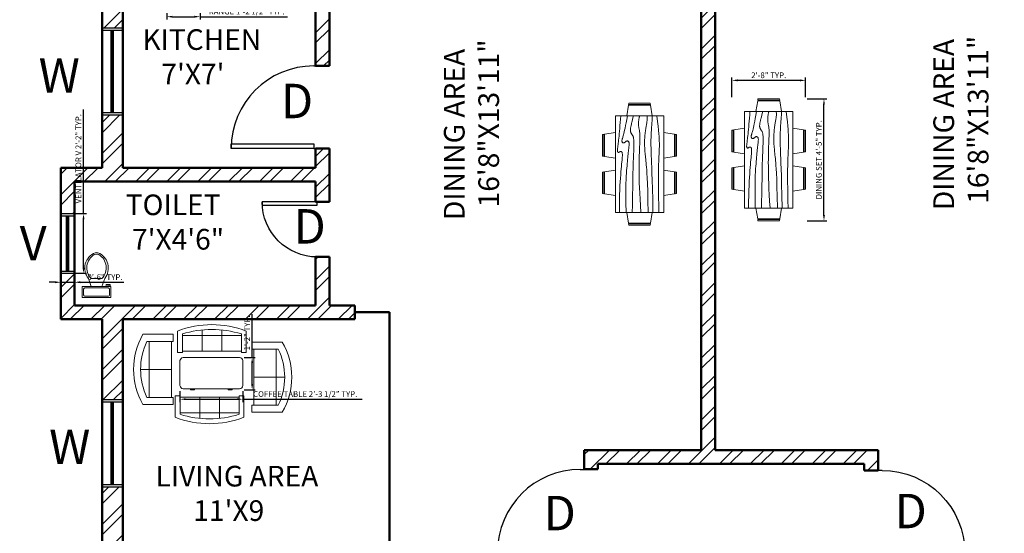
# Model space of a CAD drawing. Units: inches. Extents: x -31485 to -28799, y 18003 to 19130.
# Tile 12 of 15: x -29700 to -29271, y 18380 to 18604. Entities that reach past the tile are written whole.
import ezdxf

# ---------------------------------------------------------------- set-up
doc = ezdxf.new("R2010")
doc.units = ezdxf.units.IN
for name, color, linetype, lineweight in [('A-ANNO-DIMS', 2, 'Continuous', 18), ('A-ANNO-TEXT', 7, 'Continuous', 18), ('A-AREA-IDEN', 7, 'Continuous', 18), ('A-DOOR', 3, 'Continuous', 25), ('A-FLOR-FIXT', 9, 'Continuous', 18), ('A-FURN', 8, 'Continuous', 18), ('A-GLAZ', 4, 'Continuous', 25), ('A-WALL', 7, 'Continuous', 50), ('A-WALL-PATT', 8, 'Continuous', 13)]:
    doc.layers.add(name, color=color, linetype=linetype, lineweight=lineweight)
doc.styles.get("Standard").update_dxf_attribs({"font": 'arial.ttf'})
doc.dimstyles.new('ISO-25', dxfattribs={"dimtxt": 2.5, "dimasz": 2.5, "dimexe": 1.25, "dimexo": 0.625, "dimtad": 1, "dimdec": 0, "dimlunit": 3, "dimtxsty": 'Standard', "dimcen": 2.5, "dimadec": 0, "dimazin": 0, "dimtfac": 1, "dimtdec": 0, "dimtmove": 0, "dimatfit": 3, "dimfxl": 1, "dimarcsym": 0})

# ---------------------------------------------------------------- blocks, each defined once
blk = doc.blocks.new('*U8')
for p, q in [((0, 0), (0, -100)), ((750, 0), (750, -100))]:
    blk.add_line(p, q)
blk.add_lwpolyline([(0, 0), (0, 750), (43.75, 750), (43.75, 0)], close=True)
blk.add_arc((0, 0), 750, 0, 90)
blk = doc.blocks.new('Toilet - top')
for p, q in [((9.5, -6), (9.5, -2)), ((-10, -8.5), (-8, -8.5)), ((-10, -9.5), (-10, -8.5)), ((-7, -9.5), (-10, -9.5)), ((-8, -8.5), (-8, -8)), ((-7, -8), (-7, -9.5)), ((-4, -8), (-6, -14)), ((4, -14), (-4, -14)), ((4, -8), (6, -14))]:
    blk.add_line(p, q)
blk.add_lwpolyline([(10.5, -8), (10.5, 0), (-10.5, 0), (-10.5, -8)], close=True)
for points in [[(-9.5, -2), (-9.5, -6)], [(8.5, -1), (-8.5, -1)], [(-8.5, -7), (8.5, -7)]]:
    blk.add_lwpolyline(points)
for centre, radius, start, end in [((-8.62, -1.88), 0.884, 81.8699, 188.1301), ((-8.62, -6.12), 0.884, 171.8699, 278.1301), ((8.62, -1.88), 0.884, 351.8699, 98.1301), ((8.62, -6.12), 0.884, 261.8699, 8.1301), ((3.52, -21.58), 12.17, 141.46911, 247.97143), ((4.2, -21.82), 11.33, 136.36773, 238.94682), ((-3.52, -21.58), 12.17, 292.02843, 38.53071), ((-4.2, -21.82), 11.33, 301.05301, 43.63209), ((0, -27.88), 4, 245.73182, 294.26817), ((0, -29), 4, 254.86053, 285.13947)]:
    blk.add_arc(centre, radius, start, end)
blk = doc.blocks.new('Dining Set - 36 x 72 in.')
for p, q in [((-22.2343, 26.00059), (-23.4847, 17.99762)), ((-22.2304, 26), (-5.7608, 26)), ((-22, 27.5), (-22.1562, 26.50042)), ((-5.8416, 26.5), (-22.1534, 26.5)), ((-22, 27.5), (-6, 27.5)), ((-5.8437, 26.49966), (-6, 27.5)), ((-4.5152, 17.99762), (-5.7655, 25.99926)), ((5.7657, 26.00059), (4.5153, 17.99762)), ((5.7696, 26), (22.2392, 26)), ((6, 27.5), (5.8438, 26.50042)), ((22.1584, 26.5), (5.8466, 26.5)), ((6, 27.5), (22, 27.5)), ((22.1563, 26.49966), (22, 27.5)), ((23.4848, 17.99762), (22.2345, 25.99926)), ((36, 18), (-36, 18)), ((-36, 18), (-36, -18)), ((36, -18), (36, 18)), ((-45.5, 8), (-44.5004, 8.15617)), ((-45.5, 8), (-45.5, -8)), ((-44.5, -8.15843), (-44.5, 8.15338)), ((-44.0006, 8.23428), (-35.9976, 9.48474)), ((-44, 8.23041), (-44, -8.23915)), ((44.0006, 8.23428), (35.9976, 9.48474)), ((44, 8.23041), (44, -8.23915)), ((44.5, -8.15843), (44.5, 8.15338)), ((45.5, 8), (44.5005, 8.15617)), ((45.5, 8), (45.5, -8)), ((-44.4997, -8.15631), (-45.5, -8)), ((-35.9976, -9.48476), (-43.9993, -8.2345)), ((35.9976, -9.48476), (43.9993, -8.2345)), ((44.4997, -8.15631), (45.5, -8)), ((-36, -18), (36, -18)), ((-22.2343, -26.0006), (-23.4847, -17.99762)), ((-4.5152, -17.99762), (-5.7655, -25.99928)), ((5.7657, -26.0006), (4.5153, -17.99762)), ((23.4848, -17.99762), (22.2345, -25.99928)), ((-22.2304, -26), (-5.7608, -26)), ((-22, -27.5), (-22.1562, -26.50044)), ((-5.8416, -26.5), (-22.1534, -26.5)), ((-22, -27.5), (-6, -27.5)), ((-5.8437, -26.49967), (-6, -27.5)), ((5.7696, -26), (22.2392, -26)), ((6, -27.5), (5.8438, -26.50044)), ((22.1584, -26.5), (5.8466, -26.5)), ((6, -27.5), (22, -27.5)), ((22.1563, -26.49967), (22, -27.5))]:
    blk.add_line(p, q)
for points in [[(-36, 15), (-31.1772, 14.97754), (-26.8079, 14.91406), (-22.8538, 14.81543), (-19.276, 14.6875), (-16.0362, 14.53613), (-13.0957, 14.36718), (-10.4159, 14.18652), (-7.9583, 14), (-5.6904, 13.81315), (-3.6035, 13.63021), (-1.6954, 13.45508), (0.0365, 13.29166), (1.5945, 13.14388), (2.9811, 13.01562), (4.1988, 12.9108), (5.25, 12.83333), (6.1393, 12.78613), (6.8802, 12.76823), (7.4883, 12.77767), (7.9792, 12.8125), (8.3685, 12.87077), (8.6719, 12.95052), (8.9049, 13.0498), (9.0833, 13.16666), (9.2205, 13.29899), (9.3216, 13.44401), (9.3895, 13.59879), (9.4271, 13.76041), (9.4373, 13.92594), (9.4232, 14.09245), (9.3875, 14.257), (9.3333, 14.41666), (9.2638, 14.56917), (9.1836, 14.71484), (9.0975, 14.85465), (9.0104, 14.98958), (8.9272, 15.1206), (8.8529, 15.2487), (8.7922, 15.37483), (8.75, 15.5), (8.7305, 15.62467), (8.7344, 15.74739), (8.7617, 15.86621), (8.8125, 15.97916), (8.8867, 16.08431), (8.9844, 16.17968), (9.1055, 16.26334), (9.25, 16.33333), (9.4189, 16.38802), (9.6172, 16.42708), (9.8506, 16.45052), (10.125, 16.45833), (10.4463, 16.45052), (10.8203, 16.42708), (11.2529, 16.38802), (11.75, 16.33333), (12.3184, 16.26318), (12.9694, 16.17838), (13.7151, 16.07991), (14.5677, 15.96875), (15.5395, 15.84586), (16.6426, 15.71224), (17.8893, 15.56884), (19.2917, 15.41666), (20.859, 15.25667), (22.5879, 15.08984), (24.4721, 14.91715), (26.5052, 14.73958), (28.6809, 14.5581), (30.9929, 14.3737), (33.4347, 14.18733), (36, 14)], [(-36, 10), (-28.9766, 10.14274), (-23.1725, 10.20442), (-18.4241, 10.19775), (-14.5677, 10.13541), (-11.4399, 10.03011), (-8.877, 9.89453), (-6.7154, 9.74137), (-4.7917, 9.58333), (-2.9698, 9.43082), (-1.2246, 9.28515), (0.4415, 9.14534), (2.026, 9.01041), (3.5266, 8.87939), (4.9408, 8.7513), (6.266, 8.62516), (7.5, 8.5), (8.6411, 8.37549), (9.6914, 8.2539), (10.6538, 8.13818), (11.5312, 8.03125), (12.3267, 7.93603), (13.043, 7.85547), (13.6831, 7.79248), (14.25, 7.75), (14.7471, 7.7303), (15.1797, 7.73307), (15.5537, 7.75732), (15.875, 7.80208), (16.1494, 7.86637), (16.3828, 7.94922), (16.5811, 8.04964), (16.75, 8.16666), (16.8944, 8.29915), (17.0143, 8.44531), (17.1089, 8.60319), (17.1771, 8.77083), (17.218, 8.94629), (17.2305, 9.1276), (17.2137, 9.31282), (17.1667, 9.5), (17.0895, 9.6875), (16.987, 9.875), (16.8649, 10.0625), (16.7292, 10.25), (16.5856, 10.4375), (16.4401, 10.625), (16.2985, 10.8125), (16.1667, 11), (16.05, 11.18733), (15.9518, 11.3737), (15.8752, 11.5581), (15.8229, 11.73958), (15.798, 11.91715), (15.8034, 12.08984), (15.842, 12.25667), (15.9167, 12.41666), (16.0295, 12.56836), (16.1784, 12.70833), (16.3605, 12.83268), (16.5729, 12.9375), (16.8127, 13.01888), (17.0768, 13.07291), (17.3625, 13.0957), (17.6667, 13.08333), (17.9894, 13.03312), (18.3418, 12.94726), (18.7382, 12.82918), (19.1927, 12.68229), (19.7195, 12.51001), (20.3327, 12.31575), (21.0465, 12.10294), (21.875, 11.875), (22.8357, 11.63354), (23.959, 11.37304), (25.2786, 11.08618), (26.8282, 10.76562), (28.6414, 10.40405), (30.752, 9.99414), (33.1936, 9.52856), (36, 9)], [(-36, 5.5), (-30.7157, 5.3348), (-26.069, 5.20963), (-21.9946, 5.11767), (-18.4271, 5.05208), (-15.3009, 5.00602), (-12.5508, 4.97265), (-10.1112, 4.94515), (-7.9167, 4.91666), (-5.909, 4.88167), (-4.0586, 4.83984), (-2.3429, 4.79215), (-0.7396, 4.73958), (0.7739, 4.6831), (2.22, 4.6237), (3.6213, 4.56233), (5, 4.5), (6.373, 4.43782), (7.7344, 4.3776), (9.0723, 4.32129), (10.375, 4.27083), (11.6309, 4.22819), (12.8281, 4.19531), (13.9551, 4.17415), (15, 4.16666), (15.954, 4.17448), (16.819, 4.19791), (17.6001, 4.23698), (18.3021, 4.29166), (18.9299, 4.36198), (19.4883, 4.44791), (19.9823, 4.54948), (20.4167, 4.66666), (20.7969, 4.79899), (21.1302, 4.94401), (21.4245, 5.09879), (21.6875, 5.26041), (21.9271, 5.42594), (22.1511, 5.59245), (22.3672, 5.757), (22.5834, 5.91666), (22.8065, 6.06868), (23.0404, 6.21093), (23.2879, 6.34147), (23.5521, 6.45833), (23.8358, 6.55957), (24.142, 6.64323), (24.4735, 6.70735), (24.8334, 6.75), (25.2235, 6.76969), (25.642, 6.76692), (26.0858, 6.74267), (26.5521, 6.69791), (27.0379, 6.63362), (27.5404, 6.55078), (28.0565, 6.45036), (28.5834, 6.33333), (29.1242, 6.19987), (29.7071, 6.04687), (30.3661, 5.87044), (31.1354, 5.66666), (32.0493, 5.43164), (33.142, 5.16146), (34.4475, 4.85221), (36, 4.5)], [(-36, -1), (-30.7915, -0.6591), (-26.0195, -0.38216), (-21.6519, -0.16284), (-17.6563, 0.00521), (-14.0005, 0.12833), (-10.6523, 0.21289), (-7.5796, 0.26522), (-4.75, 0.29166), (-2.134, 0.29793), (0.2878, 0.28711), (2.5317, 0.26163), (4.6146, 0.22396), (6.5529, 0.17651), (8.3633, 0.12174), (10.0623, 0.06209), (11.6667, 0), (13.1899, -0.06201), (14.6341, -0.1211), (15.9982, -0.17432), (17.2813, -0.21875), (18.4823, -0.25147), (19.6003, -0.26953), (20.6343, -0.27002), (21.5834, -0.25), (22.4481, -0.20768), (23.2357, -0.14584), (23.9549, -0.06836), (24.6146, 0.02083), (25.2235, 0.11784), (25.7904, 0.21875), (26.3241, 0.31966), (26.8334, 0.41666), (27.3265, 0.50618), (27.8099, 0.58593), (28.2894, 0.65397), (28.7709, 0.70833), (29.2601, 0.74707), (29.763, 0.76823), (30.2855, 0.76985), (30.8334, 0.75), (31.4088, 0.70784), (31.9994, 0.64713), (32.589, 0.57275), (33.1615, 0.48958), (33.7008, 0.4025), (34.1908, 0.3164), (34.6153, 0.23616), (34.9584, 0.16666), (35.2099, 0.11165), (35.3848, 0.07031), (35.504, 0.04069), (35.5886, 0.02083), (35.6594, 0.00879), (35.7377, 0.0026), (35.8442, 0.00032), (36, 0)], [(-36, -6.5), (-27.1843, -6.31267), (-20.084, -6.1263), (-14.469, -5.9419), (-10.1094, -5.76042), (-6.7752, -5.58285), (-4.2363, -5.41016), (-2.2629, -5.24333), (-0.625, -5.08334), (0.8708, -4.93099), (2.2715, -4.78646), (3.5872, -4.64974), (4.8281, -4.52084), (6.0046, -4.39974), (7.127, -4.28646), (8.2053, -4.18099), (9.25, -4.08334), (10.2705, -3.99382), (11.2734, -3.91407), (12.2647, -3.84603), (13.25, -3.79167), (14.2354, -3.75293), (15.2266, -3.73177), (16.2295, -3.73015), (17.25, -3.75), (18.2912, -3.79248), (19.3451, -3.85547), (20.4009, -3.93604), (21.4479, -4.03125), (22.4754, -4.13819), (23.4727, -4.25391), (24.4289, -4.37549), (25.3334, -4.5), (26.1785, -4.62492), (26.9694, -4.74935), (27.7145, -4.87281), (28.4219, -4.99479), (29.1, -5.11483), (29.7572, -5.23242), (30.4016, -5.34709), (31.0417, -5.45834), (31.6837, -5.56437), (32.3262, -5.65821), (32.9658, -5.73153), (33.599, -5.77604), (34.2224, -5.78345), (34.8327, -5.74545), (35.4264, -5.65373), (36, -5.5)], [(-36, -10), (-26.4022, -9.81299), (-18.4675, -9.62891), (-11.9839, -9.45069), (-6.7396, -9.28125), (-2.5226, -9.12354), (0.8789, -8.98047), (3.6769, -8.85498), (6.0833, -8.75), (8.2767, -8.66765), (10.3021, -8.60677), (12.1712, -8.56543), (13.8958, -8.54167), (15.4876, -8.53353), (16.9583, -8.53907), (18.3197, -8.55632), (19.5834, -8.58334), (20.7616, -8.61841), (21.8685, -8.66081), (22.9188, -8.71004), (23.9271, -8.76563), (24.9081, -8.82707), (25.8763, -8.89388), (26.8465, -8.96558), (27.8334, -9.04167), (28.8474, -9.12118), (29.8828, -9.20117), (30.93, -9.27824), (31.9792, -9.34896), (33.0205, -9.40991), (34.0443, -9.45768), (35.0407, -9.48885), (36, -9.5)], [(-36, -14.5), (-30.0881, -14.33513), (-25.0332, -14.21224), (-20.7312, -14.12647), (-17.0781, -14.07292), (-13.97, -14.04671), (-11.3027, -14.04297), (-8.9724, -14.05681), (-6.875, -14.08334), (-4.9224, -14.11833), (-3.0905, -14.16016), (-1.3709, -14.20785), (0.2448, -14.26042), (1.7647, -14.3169), (3.1973, -14.3763), (4.5507, -14.43767), (5.8333, -14.5), (7.0554, -14.5621), (8.235, -14.62175), (9.3922, -14.67652), (10.5469, -14.72396), (11.7192, -14.76164), (12.929, -14.78711), (14.1965, -14.79794), (15.5417, -14.79167), (16.9933, -14.76424), (18.6152, -14.70508), (20.4804, -14.60197), (22.6615, -14.44271), (25.2312, -14.21509), (28.2624, -13.9069), (31.8277, -13.50594), (36, -13)]]:
    blk.add_lwpolyline(points)
blk = doc.blocks.new('Desk - 30 x 60 in.')
for p, q in [((-26.999995, 0), (26.999995, 0)), ((-29.999995, -27), (-29.999995, -3)), ((29.999995, -3), (29.999995, -27)), ((26.999995, -30), (-26.999995, -30)), ((-20.000005, -30), (-20.000005, -31)), ((-20.000005, -31), (-16.000005, -31)), ((-16.000005, -31), (-16.000005, -30)), ((15.999995, -31), (15.999995, -30)), ((19.999995, -31), (15.999995, -31)), ((19.999995, -30), (19.999995, -31))]:
    blk.add_line(p, q)
for centre, start, end in [((-26.499995, -3.5), 98.1301, 171.8699), ((26.499995, -3.5), 8.130102, 81.8699), ((-26.499995, -26.5), 188.1301, 261.8699), ((26.499995, -26.5), 278.1301, 351.8699)]:
    blk.add_arc(centre, 3.535534, start, end)
blk = doc.blocks.new('Sofa - Roundback 7 ft.')
for p, q in [((-36.000027, -34), (-36.000027, -11.4696)), ((-12.00002, -32.4421), (-12.00003, -6.5971)), ((11.99997, -32.4421), (11.99998, -6.5971)), ((35.99998, -34), (35.99998, -11.4696)), ((-35.999844, -13.3819), (35.9998, -13.3819)), ((-36.000027, -32.4421), (35.99998, -32.4421))]:
    blk.add_line(p, q)
for points in [[(-36.000027, -34), (-42.000027, -34), (-42.000027, -8)], [(41.99998, -8), (41.99998, -34), (35.99998, -34)]]:
    blk.add_lwpolyline(points)
for centre, radius, start, end in [((0, -114.25), 114.25, 68.43141, 111.5686), ((-0.00001, -127.1968), 121.1968, 72.72033, 107.2797)]:
    blk.add_arc(centre, radius, start, end)
blk = doc.blocks.new('Sofa - Roundback Loveseat 5 ft.')
for p, q in [((0, -32.44198), (0, -5.99998)), ((-24, -33.99998), (-24, -11.46958)), ((-23.9998, -13.38178), (23.99986, -13.38178)), ((24.00004, -33.99998), (24.00004, -11.46958)), ((-24, -32.44198), (24.00004, -32.44198))]:
    blk.add_line(p, q)
for points in [[(-24, -33.99998), (-30, -33.99998), (-30, -7.99998)], [(30.00004, -7.99998), (30.00004, -33.99998), (24.00004, -33.99998)]]:
    blk.add_lwpolyline(points)
for centre, radius, start, end in [((0, -60.24998), 60.24998, 60.13715, 119.8628), ((0, -61.38438), 55.38444, 64.32083, 115.6792)]:
    blk.add_arc(centre, radius, start, end)
blk = doc.blocks.new('WIN-900-W9')
for p, q in [((-29982.21, 18824.12), (-29982.21, 18815.12)), ((-29981.21, 18824.12), (-29981.21, 18815.12)), ((-29945.21, 18824.12), (-29945.21, 18815.12)), ((-29944.21, 18824.12), (-29944.21, 18815.12)), ((-29981.21, 18820.12), (-29945.21, 18820.12)), ((-29981.21, 18819.62), (-29945.21, 18819.62)), ((-29981.21, 18819.12), (-29945.21, 18819.12))]:
    blk.add_line(p, q)
blk = doc.blocks.new('VENT-600-W6')
for p, q in [((-29884.21, 18519.12), (-29878.21, 18519.12)), ((-29884.21, 18518.12), (-29878.21, 18518.12)), ((-29881.71, 18494.12), (-29881.71, 18518.12)), ((-29881.21, 18494.12), (-29881.21, 18518.12)), ((-29880.71, 18494.12), (-29880.71, 18518.12)), ((-29884.21, 18494.12), (-29878.21, 18494.12)), ((-29884.21, 18493.12), (-29878.21, 18493.12))]:
    blk.add_line(p, q)
blk = doc.blocks.new('*D214')
at = {"layer": 'A-ANNO-DIMS', "color": 0, "lineweight": -2, "transparency": 16777216}
for p, q in [((-29671.92, 18519.12), (-29671.92, 18564.43)), ((-29675.2, 18519.12), (-29670.67, 18519.12)), ((-29671.92, 18495.62), (-29671.92, 18516.62)), ((-29675.2, 18493.12), (-29670.67, 18493.12))]:
    blk.add_line(p, q, dxfattribs=at)
at = {"layer": 'A-ANNO-DIMS', "color": 0, "transparency": 16777216}
for points in [[(-29672.34, 18516.62), (-29671.5, 18516.62), (-29671.92, 18519.12)], [(-29672.34, 18495.62), (-29671.5, 18495.62), (-29671.92, 18493.12)]]:
    blk.add_solid(points, dxfattribs=at)
at = {"layer": 'Defpoints', "color": 0, "transparency": 16777216}
for p in [(-29675.82, 18519.12), (-29671.92, 18519.12), (-29675.82, 18493.12)]:
    blk.add_point(p, dxfattribs=at)
at = {"layer": 'A-ANNO-DIMS', "color": 0, "transparency": 16777216, "insert": (-29673.84, 18543.02), "char_height": 2.5, "attachment_point": 5, "rotation": 90}
blk.add_mtext('VENTILATOR V 2\'-2" TYP.', dxfattribs=at)
blk = doc.blocks.new('*D215')
at = {"layer": 'A-ANNO-DIMS', "color": 0, "lineweight": -2, "transparency": 16777216}
for p, q in [((-29681.82, 18492.49), (-29681.82, 18487.97)), ((-29675.82, 18492.49), (-29675.82, 18487.97)), ((-29684.32, 18489.22), (-29686.82, 18489.22)), ((-29681.82, 18489.22), (-29675.82, 18489.22)), ((-29673.32, 18489.22), (-29654.33, 18489.22))]:
    blk.add_line(p, q, dxfattribs=at)
at = {"layer": 'A-ANNO-DIMS', "color": 0, "transparency": 16777216}
for points in [[(-29684.32, 18489.63), (-29684.32, 18488.8), (-29681.82, 18489.22)], [(-29673.32, 18489.63), (-29673.32, 18488.8), (-29675.82, 18489.22)]]:
    blk.add_solid(points, dxfattribs=at)
at = {"layer": 'Defpoints', "color": 0, "transparency": 16777216}
for p in [(-29681.82, 18493.12), (-29675.82, 18493.12), (-29675.82, 18489.22)]:
    blk.add_point(p, dxfattribs=at)
at = {"layer": 'A-ANNO-DIMS', "color": 0, "transparency": 16777216, "insert": (-29662.58, 18491.12), "char_height": 2.5, "attachment_point": 5}
blk.add_mtext('0\'-6" TYP.', dxfattribs=at)
blk = doc.blocks.new('*D244')
at = {"layer": 'A-ANNO-DIMS', "color": 0, "lineweight": -2, "transparency": 16777216}
for p, q in [((-29629.9, 18441.75), (-29629.9, 18437.02)), ((-29602.57, 18441.75), (-29602.57, 18437.02)), ((-29627.4, 18438.27), (-29605.07, 18438.27)), ((-29602.57, 18438.27), (-29550.61, 18438.27))]:
    blk.add_line(p, q, dxfattribs=at)
at = {"layer": 'A-ANNO-DIMS', "color": 0, "transparency": 16777216}
for points in [[(-29627.4, 18438.69), (-29627.4, 18437.86), (-29629.9, 18438.27)], [(-29605.07, 18438.69), (-29605.07, 18437.86), (-29602.57, 18438.27)]]:
    blk.add_solid(points, dxfattribs=at)
at = {"layer": 'Defpoints', "color": 0, "transparency": 16777216}
for p in [(-29629.9, 18442.37), (-29602.57, 18442.37), (-29602.57, 18438.27)]:
    blk.add_point(p, dxfattribs=at)
at = {"layer": 'A-ANNO-DIMS', "color": 0, "transparency": 16777216, "insert": (-29575.34, 18440.19), "char_height": 2.5, "attachment_point": 5}
blk.add_mtext('COFFEE TABLE 2\'-3 1/2" TYP.', dxfattribs=at)
blk = doc.blocks.new('*D245')
at = {"layer": 'A-ANNO-DIMS', "color": 0, "lineweight": -2, "transparency": 16777216}
for p, q in [((-29598.46, 18456.5), (-29598.46, 18475.25)), ((-29601.94, 18456.5), (-29597.21, 18456.5)), ((-29598.46, 18444.87), (-29598.46, 18454)), ((-29601.94, 18442.37), (-29597.21, 18442.37))]:
    blk.add_line(p, q, dxfattribs=at)
at = {"layer": 'A-ANNO-DIMS', "color": 0, "transparency": 16777216}
for points in [[(-29598.88, 18454), (-29598.05, 18454), (-29598.46, 18456.5)], [(-29598.88, 18444.87), (-29598.05, 18444.87), (-29598.46, 18442.37)]]:
    blk.add_solid(points, dxfattribs=at)
at = {"layer": 'Defpoints', "color": 0, "transparency": 16777216}
for p in [(-29602.57, 18456.5), (-29598.46, 18456.5), (-29602.57, 18442.37)]:
    blk.add_point(p, dxfattribs=at)
at = {"layer": 'A-ANNO-DIMS', "color": 0, "transparency": 16777216, "insert": (-29600.35, 18467.13), "char_height": 2.5, "attachment_point": 5, "rotation": 90}
blk.add_mtext('1\'-2" TYP.', dxfattribs=at)
blk = doc.blocks.new('*D250')
at = {"layer": 'A-ANNO-DIMS', "color": 0, "lineweight": -2, "transparency": 16777216}
for p, q in [((-29635.69, 18606.46), (-29635.69, 18603.66)), ((-29621.14, 18606.46), (-29621.14, 18603.66)), ((-29633.19, 18604.91), (-29623.64, 18604.91)), ((-29621.14, 18604.91), (-29583.06, 18604.91))]:
    blk.add_line(p, q, dxfattribs=at)
at = {"layer": 'A-ANNO-DIMS', "color": 0, "transparency": 16777216}
for points in [[(-29633.19, 18605.32), (-29633.19, 18604.49), (-29635.69, 18604.91)], [(-29623.64, 18605.32), (-29623.64, 18604.49), (-29621.14, 18604.91)]]:
    blk.add_solid(points, dxfattribs=at)
at = {"layer": 'Defpoints', "color": 0, "transparency": 16777216}
for p in [(-29635.69, 18607.09), (-29621.14, 18607.09), (-29621.14, 18604.91)]:
    blk.add_point(p, dxfattribs=at)
at = {"layer": 'A-ANNO-DIMS', "color": 0, "transparency": 16777216, "insert": (-29600.85, 18606.82), "char_height": 2.5, "attachment_point": 5}
blk.add_mtext('RANGE 1\'-2 1/2" TYP.', dxfattribs=at)
blk = doc.blocks.new('*D262')
at = {"layer": 'A-ANNO-DIMS', "color": 0, "lineweight": -2, "transparency": 16777216}
for p, q in [((-29356.73, 18569.18), (-29348.13, 18569.18)), ((-29349.38, 18518.47), (-29349.38, 18566.68)), ((-29356.73, 18515.97), (-29348.13, 18515.97))]:
    blk.add_line(p, q, dxfattribs=at)
at = {"layer": 'A-ANNO-DIMS', "color": 0, "transparency": 16777216}
for points in [[(-29349.79, 18566.68), (-29348.96, 18566.68), (-29349.38, 18569.18)], [(-29349.79, 18518.47), (-29348.96, 18518.47), (-29349.38, 18515.97)]]:
    blk.add_solid(points, dxfattribs=at)
at = {"layer": 'Defpoints', "color": 0, "transparency": 16777216}
for p in [(-29357.36, 18569.18), (-29349.38, 18569.18), (-29357.36, 18515.97)]:
    blk.add_point(p, dxfattribs=at)
at = {"layer": 'A-ANNO-DIMS', "color": 0, "transparency": 16777216, "insert": (-29351.3, 18542.58), "char_height": 2.5, "attachment_point": 5, "rotation": 90}
blk.add_mtext('DINING SET 4\'-5" TYP.', dxfattribs=at)
blk = doc.blocks.new('*D263')
at = {"layer": 'A-ANNO-DIMS', "color": 0, "lineweight": -2, "transparency": 16777216}
for p, q in [((-29389.52, 18569.81), (-29389.52, 18578.42)), ((-29359.86, 18577.17), (-29387.02, 18577.17)), ((-29357.36, 18569.81), (-29357.36, 18578.42))]:
    blk.add_line(p, q, dxfattribs=at)
at = {"layer": 'A-ANNO-DIMS', "color": 0, "transparency": 16777216}
for points in [[(-29387.02, 18577.58), (-29387.02, 18576.75), (-29389.52, 18577.17)], [(-29359.86, 18577.58), (-29359.86, 18576.75), (-29357.36, 18577.17)]]:
    blk.add_solid(points, dxfattribs=at)
at = {"layer": 'Defpoints', "color": 0, "transparency": 16777216}
for p in [(-29389.52, 18577.17), (-29389.52, 18569.18), (-29357.36, 18569.18)]:
    blk.add_point(p, dxfattribs=at)
at = {"layer": 'A-ANNO-DIMS', "color": 0, "transparency": 16777216, "insert": (-29373.44, 18579.07), "char_height": 2.5, "attachment_point": 5}
blk.add_mtext('2\'-8" TYP.', dxfattribs=at)

msp = doc.modelspace()

# ---------------------------------------------------------------- hatches: boundary and pattern name
at = {"layer": 'A-WALL-PATT'}
h = msp.add_hatch(dxfattribs=at)
h.set_pattern_fill('ANSI32', color=256)
h.set_pattern_definition([(45, (-227.67, 0), (-6.735192, 6.735192), []), (45, (-223.18, 0), (-6.735192, 6.735192), [])])
h.paths.add_polyline_path([(-29507.82, 18213.12), (-29493.82, 18213.12), (-29493.82, 18219.12), (-29507.82, 18219.12), (-29507.82, 18309.12), (-29504.3, 18309.12), (-29504.3, 18315.12), (-29513.82, 18315.12), (-29513.82, 18243.12), (-29654.82, 18243.12), (-29654.82, 18265.36), (-29663.82, 18265.36), (-29663.82, 18180.12), (-29603.32, 18180.12), (-29603.32, 18189.12), (-29654.82, 18189.12), (-29654.82, 18237.12), (-29513.82, 18237.12), (-29513.82, 18189.12), (-29565.32, 18189.12), (-29565.32, 18180.12), (-29507.82, 18180.12)])
h.paths.add_polyline_path([(-29408.82, 18189.12), (-29447.82, 18189.12), (-29447.82, 18371.74), (-29453.82, 18371.74), (-29453.82, 18365.12), (-29476.66, 18365.12), (-29476.66, 18359.12), (-29453.82, 18359.12), (-29453.82, 18315.12), (-29480.3, 18315.12), (-29480.3, 18309.12), (-29453.82, 18309.12), (-29453.82, 18219.12), (-29467.82, 18219.12), (-29467.82, 18213.12), (-29453.82, 18213.12), (-29453.82, 18180.12), (-29408.82, 18180.12)])
h.paths.add_polyline_path([(-29325.82, 18213.12), (-29311.82, 18213.12), (-29311.82, 18219.12), (-29325.82, 18219.12), (-29325.82, 18309.12), (-29298.35, 18309.12), (-29298.35, 18315.12), (-29325.82, 18315.12), (-29325.82, 18359.12), (-29304.41, 18359.12), (-29304.41, 18365.12), (-29325.82, 18365.12), (-29325.82, 18371.25), (-29331.82, 18371.25), (-29331.82, 18189.12), (-29370.82, 18189.12), (-29370.82, 18180.12), (-29325.82, 18180.12)])
h.paths.add_polyline_path([(-29265.82, 18237.12), (-29124.82, 18237.12), (-29124.82, 18189.12), (-29176.32, 18189.12), (-29176.32, 18180.12), (-29115.82, 18180.12), (-29115.82, 18268.84), (-29124.82, 18268.84), (-29124.82, 18243.12), (-29265.82, 18243.12), (-29265.82, 18315.12), (-29274.35, 18315.12), (-29274.35, 18309.12), (-29271.82, 18309.12), (-29271.82, 18219.12), (-29285.82, 18219.12), (-29285.82, 18213.12), (-29271.82, 18213.12), (-29271.82, 18180.12), (-29214.32, 18180.12), (-29214.32, 18189.12), (-29265.82, 18189.12)])
h.paths.add_polyline_path([(-29209.82, 18365.12), (-29262.82, 18365.12), (-29268.41, 18365.12), (-29268.41, 18359.12), (-29209.82, 18359.12)])
h.paths.add_polyline_path([(-29085.82, 18365.12), (-29115.82, 18365.12), (-29115.82, 18400.12), (-29124.82, 18400.12), (-29124.82, 18365.12), (-29171.82, 18365.12), (-29171.82, 18359.12), (-29124.82, 18359.12), (-29124.82, 18306.84), (-29115.82, 18306.84), (-29115.82, 18317.12), (-29085.82, 18317.12)])
h.paths.add_polyline_path([(-29115.82, 18359.12), (-29091.82, 18359.12), (-29091.82, 18323.12), (-29115.82, 18323.12)], flags=16)
h.paths.add_polyline_path([(-29607.82, 18365.12), (-29654.82, 18365.12), (-29654.82, 18400.12), (-29663.82, 18400.12), (-29663.82, 18365.12), (-29693.82, 18365.12), (-29693.82, 18317.12), (-29663.82, 18317.12), (-29663.82, 18303.36), (-29654.82, 18303.36), (-29654.82, 18359.12), (-29607.82, 18359.12)])
h.paths.add_polyline_path([(-29663.82, 18359.12), (-29663.82, 18323.12), (-29687.82, 18323.12), (-29687.82, 18359.12)], flags=16)
h.paths.add_polyline_path([(-29512.66, 18365.12), (-29516.82, 18365.12), (-29569.82, 18365.12), (-29569.82, 18359.12), (-29512.66, 18359.12)])
h.paths.add_polyline_path([(-29654.82, 18473.12), (-29553.73, 18473.12), (-29553.73, 18479.12), (-29564.82, 18479.12), (-29564.82, 18500.25), (-29569.57, 18500.25, -0.011537), (-29570.67, 18500.25), (-29570.82, 18500.25), (-29570.82, 18479.12), (-29675.82, 18479.12), (-29675.82, 18493.12), (-29681.82, 18493.12), (-29681.82, 18473.12), (-29663.82, 18473.12), (-29663.82, 18438.12), (-29654.82, 18438.12)])
h.paths.add_polyline_path([(-29564.82, 18547.44), (-29570.82, 18547.44), (-29570.82, 18539.12), (-29654.82, 18539.12), (-29654.82, 18562.12), (-29663.82, 18562.12), (-29663.82, 18539.12), (-29681.82, 18539.12), (-29681.82, 18519.12), (-29675.82, 18519.12), (-29675.82, 18533.12), (-29570.82, 18533.12), (-29570.82, 18524.25), (-29564.82, 18524.25)])
h.paths.add_polyline_path([(-29563.19, 18629.12), (-29654.82, 18629.12), (-29654.82, 18682.12), (-29663.82, 18682.12), (-29663.82, 18600.12), (-29654.82, 18600.12), (-29654.82, 18623.12), (-29570.82, 18623.12), (-29570.82, 18583.44), (-29566.85, 18583.44), (-29564.82, 18583.44), (-29564.82, 18623.12), (-29563.19, 18623.12)])
h.paths.add_polyline_path([(-29315.33, 18629.12), (-29396.82, 18629.12), (-29396.82, 18682.12), (-29402.82, 18682.12), (-29402.82, 18629.12), (-29482.28, 18629.12), (-29482.28, 18626.12), (-29482.28, 18623.12), (-29402.82, 18623.12), (-29402.82, 18416.12), (-29453.82, 18416.12), (-29453.82, 18407.74), (-29447.82, 18407.74), (-29447.82, 18410.12), (-29331.82, 18410.12), (-29331.82, 18407.25), (-29325.82, 18407.25), (-29325.82, 18416.12), (-29396.82, 18416.12), (-29396.82, 18623.12), (-29315.33, 18623.12)])
h.paths.add_polyline_path([(-29525.82, 18773.12), (-29492.32, 18773.12), (-29492.32, 18779.12), (-29498.82, 18779.12), (-29498.82, 18815.12), (-29469.82, 18815.12), (-29469.82, 18824.12), (-29504.82, 18824.12), (-29504.82, 18779.12), (-29552.82, 18779.12), (-29552.82, 18824.12), (-29587.82, 18824.12), (-29587.82, 18815.12), (-29558.82, 18815.12), (-29558.82, 18779.12), (-29563.08, 18779.12), (-29563.08, 18776.12), (-29563.08, 18773.12), (-29531.82, 18773.12), (-29531.82, 18629.12), (-29533.3, 18629.12), (-29533.3, 18626.12), (-29533.3, 18623.12), (-29518.28, 18623.12), (-29518.28, 18629.12), (-29525.82, 18629.12)])
h.paths.add_polyline_path([(-29654.82, 18779.12), (-29654.82, 18815.12), (-29625.82, 18815.12), (-29625.82, 18824.12), (-29663.82, 18824.12), (-29663.82, 18779.12), (-29693.82, 18779.12), (-29693.82, 18731.12), (-29663.82, 18731.12), (-29663.82, 18720.12), (-29654.82, 18720.12), (-29654.82, 18773.12), (-29587.08, 18773.12), (-29587.08, 18779.12)])
h.paths.add_polyline_path([(-29663.82, 18773.12), (-29663.82, 18737.12), (-29687.82, 18737.12), (-29687.82, 18773.12)], flags=16)
h.paths.add_polyline_path([(-29396.82, 18815.12), (-29367.82, 18815.12), (-29367.82, 18824.12), (-29431.82, 18824.12), (-29431.82, 18815.12), (-29402.82, 18815.12), (-29402.82, 18779.12), (-29468.32, 18779.12), (-29468.32, 18776.12), (-29468.32, 18773.12), (-29402.82, 18773.12), (-29402.82, 18720.12), (-29396.82, 18720.12), (-29396.82, 18773.12), (-29331.17, 18773.12), (-29331.17, 18779.12), (-29396.82, 18779.12)])
h.paths.add_polyline_path([(-29232.68, 18779.12), (-29240.82, 18779.12), (-29240.82, 18815.12), (-29201.82, 18815.12), (-29201.82, 18824.12), (-29246.82, 18824.12), (-29246.82, 18779.12), (-29294.82, 18779.12), (-29294.82, 18824.12), (-29329.82, 18824.12), (-29329.82, 18815.12), (-29300.82, 18815.12), (-29300.82, 18779.12), (-29307.17, 18779.12), (-29307.17, 18776.12), (-29307.17, 18773.12), (-29273.82, 18773.12), (-29273.82, 18629.12), (-29279.33, 18629.12), (-29279.33, 18626.12), (-29279.33, 18623.12), (-29262.04, 18623.12), (-29262.04, 18629.12), (-29267.82, 18629.12), (-29267.82, 18773.12), (-29232.68, 18773.12)])
h.paths.add_polyline_path([(-29085.82, 18779.12), (-29115.82, 18779.12), (-29115.82, 18824.12), (-29163.82, 18824.12), (-29163.82, 18815.12), (-29124.82, 18815.12), (-29124.82, 18779.12), (-29208.68, 18779.12), (-29208.68, 18776.12), (-29208.68, 18773.12), (-29124.82, 18773.12), (-29124.82, 18720.12), (-29115.82, 18720.12), (-29115.82, 18731.12), (-29085.82, 18731.12)])
h.paths.add_polyline_path([(-29115.82, 18773.12), (-29091.82, 18773.12), (-29091.82, 18737.12), (-29115.82, 18737.12)], flags=16)
h.paths.add_polyline_path([(-29115.82, 18682.12), (-29124.82, 18682.12), (-29124.82, 18629.12), (-29226.04, 18629.12), (-29226.04, 18626.12), (-29226.04, 18623.12), (-29214.82, 18623.12), (-29214.82, 18589.35), (-29208.82, 18589.35), (-29208.82, 18623.12), (-29124.82, 18623.12), (-29124.82, 18600.12), (-29115.82, 18600.12)])
h.paths.add_polyline_path([(-29115.82, 18562.12), (-29124.82, 18562.12), (-29124.82, 18539.12), (-29208.82, 18539.12), (-29208.82, 18553.35), (-29211.82, 18553.35), (-29214.82, 18553.35), (-29214.82, 18522.99), (-29208.82, 18522.99), (-29208.82, 18533.12), (-29103.82, 18533.12), (-29103.82, 18519.12), (-29097.82, 18519.12), (-29097.82, 18539.12), (-29115.82, 18539.12)])
h.paths.add_polyline_path([(-29115.82, 18473.12), (-29097.82, 18473.12), (-29097.82, 18493.12), (-29103.82, 18493.12), (-29103.82, 18479.12), (-29208.82, 18479.12), (-29208.82, 18498.99), (-29214.82, 18498.99), (-29214.82, 18479.12), (-29238.82, 18479.12), (-29238.82, 18473.12), (-29124.82, 18473.12), (-29124.82, 18438.12), (-29115.82, 18438.12)])
h.paths.add_polyline_path([(-29513.85, 18245.24), (-29448.79, 18245.24), (-29448.79, 18278.82), (-29513.85, 18278.82)], flags=9)
h.paths.add_polyline_path([(-29331.85, 18241.25), (-29266.79, 18241.25), (-29266.79, 18274.84), (-29331.85, 18274.84)], flags=9)
h.paths.add_polyline_path([(-29095.1, 18330.99), (-29095.1, 18356.44), (-29113.65, 18356.44), (-29113.65, 18330.99)], flags=8)
h.paths.add_polyline_path([(-29666.32, 18333.81), (-29666.32, 18359.25), (-29684.87, 18359.25), (-29684.87, 18333.81)], flags=24)
h.paths.add_polyline_path([(-29665.76, 18745.92), (-29665.76, 18771.37), (-29684.31, 18771.37), (-29684.31, 18745.92)], flags=8)
h.paths.add_polyline_path([(-29093.62, 18744.62), (-29093.62, 18770.06), (-29112.17, 18770.06), (-29112.17, 18744.62)], flags=8)

# ---------------------------------------------------------------- linework, layer by layer
at = {"layer": 'A-WALL'}
for p, q in [((-29663.82, 18539.12), (-29663.82, 18731.12)), ((-29654.82, 18539.12), (-29654.82, 18623.12)), ((-29570.82, 18583.44), (-29570.82, 18623.12)), ((-29564.82, 18583.44), (-29564.82, 18623.12)), ((-29402.82, 18416.12), (-29402.82, 18623.12)), ((-29396.82, 18416.12), (-29396.82, 18623.12)), ((-29570.82, 18583.44), (-29564.82, 18583.44)), ((-29570.82, 18539.12), (-29570.82, 18547.44)), ((-29570.82, 18547.44), (-29564.82, 18547.44)), ((-29564.82, 18524.25), (-29564.82, 18547.44)), ((-29681.82, 18539.12), (-29663.82, 18539.12)), ((-29681.82, 18473.12), (-29681.82, 18539.12)), ((-29654.82, 18539.12), (-29570.82, 18539.12)), ((-29675.82, 18533.12), (-29570.82, 18533.12)), ((-29675.82, 18479.12), (-29675.82, 18533.12)), ((-29570.82, 18524.25), (-29570.82, 18533.12)), ((-29570.82, 18524.25), (-29564.82, 18524.25)), ((-29570.82, 18479.12), (-29570.82, 18500.25)), ((-29570.82, 18500.25), (-29564.82, 18500.25)), ((-29564.82, 18479.12), (-29564.82, 18500.25)), ((-29675.82, 18479.12), (-29570.82, 18479.12)), ((-29564.82, 18479.12), (-29553.73, 18479.12)), ((-29553.73, 18479.12), (-29553.73, 18473.12)), ((-29681.82, 18473.12), (-29663.82, 18473.12)), ((-29663.82, 18365.12), (-29663.82, 18473.12)), ((-29654.82, 18365.12), (-29654.82, 18473.12)), ((-29654.82, 18473.12), (-29553.73, 18473.12)), ((-29553.73, 18476.12), (-29538.64, 18476.12)), ((-29538.64, 18476.12), (-29538.64, 18365.12)), ((-29402.82, 18416.12), (-29453.82, 18416.12)), ((-29453.82, 18407.74), (-29453.82, 18416.12)), ((-29325.82, 18416.12), (-29396.82, 18416.12)), ((-29325.82, 18416.12), (-29325.82, 18407.25)), ((-29331.82, 18410.12), (-29447.82, 18410.12)), ((-29447.82, 18407.74), (-29447.82, 18410.12)), ((-29331.82, 18410.12), (-29331.82, 18407.25)), ((-29453.82, 18407.74), (-29447.82, 18407.74)), ((-29331.82, 18407.25), (-29325.82, 18407.25))]:
    msp.add_line(p, q, dxfattribs=at)

# ---------------------------------------------------------------- block references
at = {"layer": 'A-DOOR'}
for p, xscale, yscale, zscale, rotation in [((-29571.65, 18547.44), 0.0480000000000013, 0.0480000000000013, 0.0480000000000013, 90.00000000000003), ((-29570.12, 18524.25), -0.0320150051253172, 0.0320150051253172, 0.0320150051253172, 90), ((-29455.56, 18371.7), 0.0480000000000013, 0.0480000000000013, 0.0480000000000013, 90.00000000000003), ((-29324.02, 18371.25), -0.0480000007307817, 0.0480000007307817, 0.0480000007307817, 270)]:
    msp.add_blockref('*U8', p, dxfattribs=dict(at, xscale=xscale, yscale=yscale, zscale=zscale, rotation=rotation))
at = {"layer": 'A-FLOR-FIXT', "xscale": 0.5926017901613329, "yscale": 0.5926017901613329, "zscale": 0.5926017901613329, "rotation": 180}
msp.add_blockref('Toilet - top', (-29666.24, 18482.59), dxfattribs=at)
at = {"layer": 'A-FURN'}
for name, p, xscale, yscale, zscale, rotation in [('Dining Set - 36 x 72 in.', (-29429.73, 18540.69), 0.5847537378471955, 0.5847537378471955, 0.5847537378471955, 90), ('Dining Set - 36 x 72 in.', (-29373.44, 18542.58), 0.5847537378471955, 0.5847537378471955, 0.5847537378471955, 90), ('Sofa - Roundback Loveseat 5 ft.', (-29650.12, 18451.25), 0.5093827995121489, 0.5093827995121489, 0.5093827995121489, 89.99999999999999), ('Sofa - Roundback Loveseat 5 ft.', (-29581.24, 18447.86), 0.5093827995121489, 0.5093827995121489, 0.5093827995121489, 270), ('Sofa - Roundback 7 ft.', (-29617.02, 18427.59), 0.356964146635117, 0.356964146635117, 0.356964146635117, 180)]:
    msp.add_blockref(name, p, dxfattribs=dict(at, xscale=xscale, yscale=yscale, zscale=zscale, rotation=rotation))
for name, p, xscale, yscale, zscale in [('Sofa - Roundback 7 ft.', (-29616.01, 18470.77), 0.356964146635117, 0.356964146635117, 0.356964146635117), ('Desk - 30 x 60 in.', (-29616.23, 18456.5), 0.4556329481741908, 0.4556329481741908, 0.4556329481741908)]:
    msp.add_blockref(name, p, dxfattribs=dict(at, xscale=xscale, yscale=yscale, zscale=zscale))
at = {"layer": 'A-GLAZ'}
for p, rotation in [((-10839.7, 48544.32), 89.9999999999743), ((-10839.7, 48382.32), 89.9999999999847)]:
    msp.add_blockref('WIN-900-W9', p, dxfattribs=dict(at, rotation=rotation))
msp.add_blockref('VENT-600-W6', (202.38, 0), dxfattribs=at)

# ---------------------------------------------------------------- texts
at = {"layer": 'A-ANNO-TEXT', "char_height": 15, "attachment_point": 1}
for s, insert in [('{W}', (-29691.48, 18586.78)), ('{D}', (-29585.98, 18575.68)), ('{D}', (-29580.47, 18521.06)), ('{V}', (-29699.74, 18513.76)), ('{W}', (-29686.92, 18425.05)), ('{D}', (-29471.55, 18396.14)), ('{D}', (-29318.66, 18397.04))]:
    msp.add_mtext_dynamic_manual_height_columns(s, width=1534.0875, gutter_width=12.5, heights=[0], dxfattribs=dict(at, insert=insert))
at = {"layer": 'A-AREA-IDEN', "char_height": 9, "attachment_point": 1}
for s, insert in [("{ KITCHEN\\P    7'X7'}", (-29649.02, 18599.45)), ('{     TOILET\\P      7\'X4\'6"}', (-29667.3, 18527.45)), ("{LIVING AREA\\P      11'X9}", (-29640.59, 18409.24))]:
    msp.add_mtext_dynamic_manual_height_columns(s, width=988.498, gutter_width=12.5, heights=[0], dxfattribs=dict(at, insert=insert))
at = {"layer": 'A-AREA-IDEN', "char_height": 9, "attachment_point": 1, "rotation": 90}
for s, insert in [('{DINING AREA\\P  16\'8"X13\'11"}', (-29514.92, 18516.32)), ('{DINING AREA\\P 16\'8"X13\'11"}', (-29301.72, 18520.64))]:
    msp.add_mtext_dynamic_manual_height_columns(s, width=988.498, gutter_width=12.5, heights=[0], dxfattribs=dict(at, insert=insert))

# ---------------------------------------------------------------- dimensions: what is measured, and where the dimension line sits
at = {"layer": 'A-ANNO-DIMS'}
for base, p1, p2, text, picture, middle in [((-29621.1354, 18604.905), (-29635.6927, 18607.0886), (-29621.1354, 18607.0886), 'RANGE <> TYP.', '*D250', (-29600.8481, 18606.8226)), ((-29675.82, 18489.22), (-29681.82, 18493.12), (-29675.82, 18493.12), '<> TYP.', '*D215', (-29662.58, 18491.12)), ((-29602.57, 18438.27), (-29629.9, 18442.37), (-29602.57, 18442.37), 'COFFEE TABLE <> TYP.', '*D244', (-29575.34, 18440.19))]:
    dim = msp.add_linear_dim(base=base, p1=p1, p2=p2, text=text, dimstyle='ISO-25', override={"dimdec": 1, "dimlfac": 1, "dimrnd": 0, "dimzin": 1, "dimdsep": 46, "dimlunit": 4, "dimfrac": 2}, dxfattribs=at)
    dim.commit()
    dim.dimension.update_dxf_attribs({"geometry": picture, "text_midpoint": middle})
for base, p1, p2, angle, text, picture, middle in [((-29389.52, 18577.17), (-29357.36, 18569.18), (-29389.52, 18569.18), 180, '<> TYP.', '*D263', (-29373.44, 18579.07)), ((-29349.38, 18569.18), (-29357.36, 18515.97), (-29357.36, 18569.18), 90, 'DINING SET <> TYP.', '*D262', (-29351.3, 18542.58)), ((-29671.92, 18519.12), (-29675.82, 18493.12), (-29675.82, 18519.12), 90, 'VENTILATOR V <> TYP.', '*D214', (-29673.84, 18543.02)), ((-29598.46, 18456.5), (-29602.57, 18442.37), (-29602.57, 18456.5), 90, '<> TYP.', '*D245', (-29600.35, 18467.13))]:
    dim = msp.add_linear_dim(base=base, p1=p1, p2=p2, angle=angle, text=text, dimstyle='ISO-25', override={"dimdec": 1, "dimlfac": 1, "dimrnd": 0, "dimzin": 1, "dimdsep": 46, "dimlunit": 4, "dimfrac": 2}, dxfattribs=at)
    dim.commit()
    dim.dimension.update_dxf_attribs({"geometry": picture, "text_midpoint": middle})

doc.saveas('drawing.dxf')
